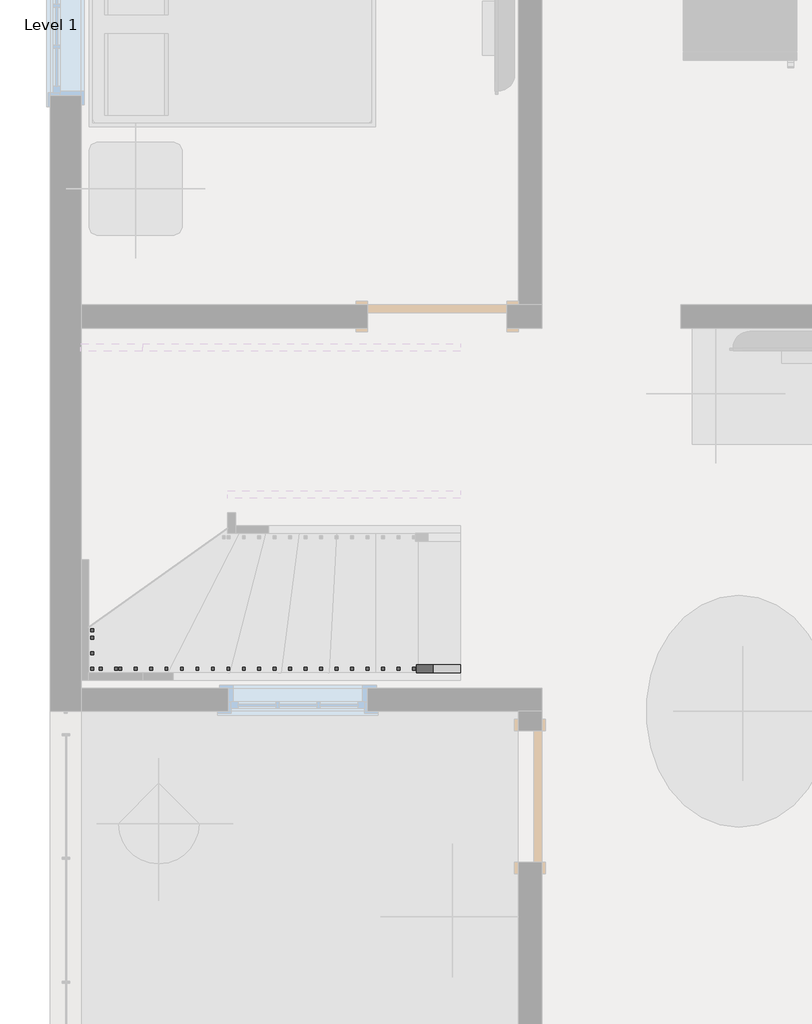
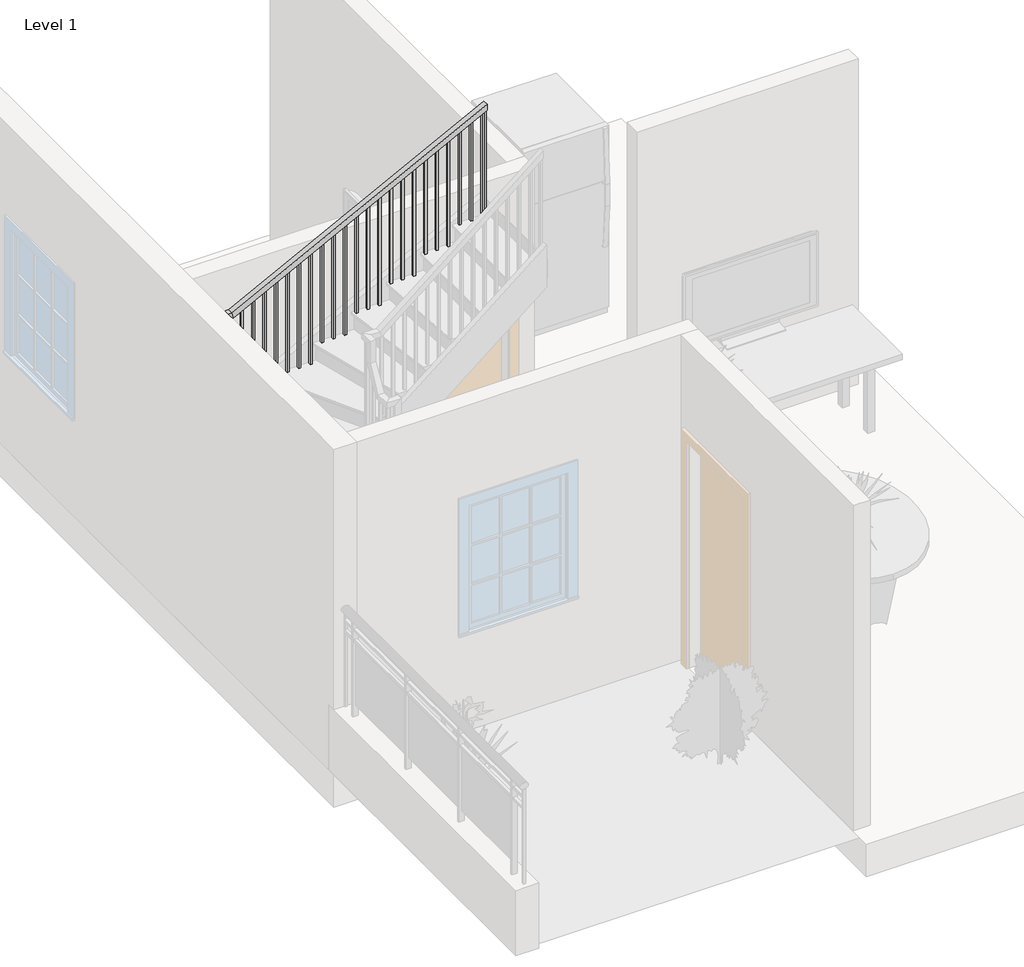
# One storey, part 2 of 3: 1 railing.
"""IFC4 building model written with IfcOpenShell, lengths in millimetres."""

from ifc_helpers import new_model, si_unit, frame, origin, place, context, project, spatial, polyline, outline, extrude, faceted_brep, element, save

model = new_model("IFC4")

# Units and contexts
model_context = context("Model", 3, world=origin())
ifc_project = project(units=[si_unit("LENGTHUNIT", "METRE", prefix="MILLI")], contexts=[model_context])

# Site, building, storey
site = spatial("IfcSite", under=ifc_project)
building = spatial("IfcBuilding", under=site)
storey = spatial("IfcBuildingStorey", under=building, Name="Level 1", Elevation=0.0)

# Railing
placement = place(None, origin())
element("IfcRailing", 1, ObjectType="Handrail - Rectangular", at=placement, inside=storey, context=model_context, shape_type="SolidModel", body=[
    faceted_brep([(-14092.4170266, 6866.6465295, 1109.0771751), (-14092.4170266, 6866.6465295, 1051.9280057), (-14092.4170266, 6917.4465295, 1051.9280057), (-14092.4170266, 6917.4465295, 1109.0771751), (-16352.3988831, 6866.6465295, 2273.7644996), (-16364.7189344, 6866.6465295, 2222.9644996), (-16364.7189344, 6917.4465295, 2222.9644996), (-16352.3988831, 6917.4465295, 2273.7644996), (-16534.5487184, 6866.6465295, 2273.7644996), (-16534.5487184, 6866.6465295, 2222.9644996), (-16483.7487184, 6917.4465295, 2222.9644996), (-16483.7487184, 6917.4465295, 2273.7644996), (-16534.5487184, 7143.8004821, 2273.7644996), (-16534.5487184, 7151.7510582, 2222.9644996), (-16483.7487184, 7151.7510582, 2222.9644996), (-16483.7487184, 7143.8004821, 2273.7644996), (-16534.5487184, 8697.6925768, 2772.3688337), (-16534.5487184, 8705.643153, 2721.5688337), (-16483.7487184, 8705.643153, 2721.5688337), (-16483.7487184, 8697.6925768, 2772.3688337), (-16534.5487184, 8974.8465295, 2772.3688337), (-16534.5487184, 8974.8465295, 2721.5688337), (-16483.7487184, 8924.0465295, 2721.5688337), (-16483.7487184, 8924.0465295, 2772.3688337), (-16352.3988831, 8974.8465295, 2772.3688337), (-16340.0788318, 8974.8465295, 2721.5688337), (-16340.0788318, 8924.0465295, 2721.5688337), (-16352.3988831, 8924.0465295, 2772.3688337), (-14092.4170266, 8974.8465295, 3937.0561582), (-14092.4170266, 8924.0465295, 3937.0561582), (-14092.4170266, 8924.0465295, 3879.9069889), (-14092.4170266, 8974.8465295, 3879.9069889)], [[[0, 1, 2, 3]], [[1, 0, 4, 5]], [[2, 1, 5, 6]], [[3, 2, 6, 7]], [[0, 3, 7, 4]], [[5, 4, 8, 9]], [[6, 5, 9, 10]], [[7, 6, 10, 11]], [[4, 7, 11, 8]], [[9, 8, 12, 13]], [[10, 9, 13, 14]], [[11, 10, 14, 15]], [[8, 11, 15, 12]], [[13, 12, 16, 17]], [[14, 13, 17, 18]], [[15, 14, 18, 19]], [[12, 15, 19, 16]], [[17, 16, 20, 21]], [[18, 17, 21, 22]], [[19, 18, 22, 23]], [[16, 19, 23, 20]], [[21, 20, 24, 25]], [[22, 21, 25, 26]], [[23, 22, 26, 27]], [[20, 23, 27, 24]], [[28, 29, 30, 31]], [[25, 24, 28, 31]], [[26, 25, 31, 30]], [[27, 26, 30, 29]], [[24, 27, 29, 28]]]),
    extrude(outline(polyline([(3862.2268642, -14126.7238831), (2878.6666667, -14126.7238831), (2878.6666667, -14107.6738831), (3872.0443296, -14107.6738831), (3862.2268642, -14126.7238831)])), frame((0.0, 8939.9215295, 0.0), z_axis=(0.0, 1.0, 0.0), x_axis=(0.0, 0.0, 1.0)), (0.0, 0.0, 1.0), 19.05),
    extrude(outline(polyline([(3809.8670491, -14228.3238831), (2878.6666667, -14228.3238831), (2878.6666667, -14209.2738831), (3819.6845145, -14209.2738831), (3809.8670491, -14228.3238831)])), frame((0.0, 8939.9215295, 0.0), z_axis=(0.0, 1.0, 0.0), x_axis=(0.0, 0.0, 1.0)), (0.0, 0.0, 1.0), 19.05),
    extrude(outline(polyline([(3757.507234, -14329.9238831), (2878.6666667, -14329.9238831), (2878.6666667, -14310.8738831), (3767.3246993, -14310.8738831), (3757.507234, -14329.9238831)])), frame((0.0, 8939.9215295, 0.0), z_axis=(0.0, 1.0, 0.0), x_axis=(0.0, 0.0, 1.0)), (0.0, 0.0, 1.0), 19.05),
    extrude(outline(polyline([(3705.1474189, -14431.5238831), (2709.3333333, -14431.5238831), (2709.3333333, -14412.4738831), (3714.9648842, -14412.4738831), (3705.1474189, -14431.5238831)])), frame((0.0, 8939.9215295, 0.0), z_axis=(0.0, 1.0, 0.0), x_axis=(0.0, 0.0, 1.0)), (0.0, 0.0, 1.0), 19.05),
    extrude(outline(polyline([(3652.7876038, -14533.1238831), (2709.3333333, -14533.1238831), (2709.3333333, -14514.0738831), (3662.6050691, -14514.0738831), (3652.7876038, -14533.1238831)])), frame((0.0, 8939.9215295, 0.0), z_axis=(0.0, 1.0, 0.0), x_axis=(0.0, 0.0, 1.0)), (0.0, 0.0, 1.0), 19.05),
    extrude(outline(polyline([(3600.4277887, -14634.7238831), (2709.3333333, -14634.7238831), (2709.3333333, -14615.6738831), (3610.245254, -14615.6738831), (3600.4277887, -14634.7238831)])), frame((0.0, 8939.9215295, 0.0), z_axis=(0.0, 1.0, 0.0), x_axis=(0.0, 0.0, 1.0)), (0.0, 0.0, 1.0), 19.05),
    extrude(outline(polyline([(3548.0679735, -14736.3238831), (2540.0, -14736.3238831), (2540.0, -14717.2738831), (3557.8854389, -14717.2738831), (3548.0679735, -14736.3238831)])), frame((0.0, 8939.9215295, 0.0), z_axis=(0.0, 1.0, 0.0), x_axis=(0.0, 0.0, 1.0)), (0.0, 0.0, 1.0), 19.05),
    extrude(outline(polyline([(3495.7081584, -14837.9238831), (2540.0, -14837.9238831), (2540.0, -14818.8738831), (3505.5256238, -14818.8738831), (3495.7081584, -14837.9238831)])), frame((0.0, 8939.9215295, 0.0), z_axis=(0.0, 1.0, 0.0), x_axis=(0.0, 0.0, 1.0)), (0.0, 0.0, 1.0), 19.05),
    extrude(outline(polyline([(3443.3483433, -14939.5238831), (2540.0, -14939.5238831), (2540.0, -14920.4738831), (3453.1658086, -14920.4738831), (3443.3483433, -14939.5238831)])), frame((0.0, 8939.9215295, 0.0), z_axis=(0.0, 1.0, 0.0), x_axis=(0.0, 0.0, 1.0)), (0.0, 0.0, 1.0), 19.05),
    extrude(outline(polyline([(3390.9885282, -15041.1238831), (2370.6666667, -15041.1238831), (2370.6666667, -15022.0738831), (3400.8059935, -15022.0738831), (3390.9885282, -15041.1238831)])), frame((0.0, 8939.9215295, 0.0), z_axis=(0.0, 1.0, 0.0), x_axis=(0.0, 0.0, 1.0)), (0.0, 0.0, 1.0), 19.05),
    extrude(outline(polyline([(3338.6287131, -15142.7238831), (2370.6666667, -15142.7238831), (2370.6666667, -15123.6738831), (3348.4461784, -15123.6738831), (3338.6287131, -15142.7238831)])), frame((0.0, 8939.9215295, 0.0), z_axis=(0.0, 1.0, 0.0), x_axis=(0.0, 0.0, 1.0)), (0.0, 0.0, 1.0), 19.05),
    extrude(outline(polyline([(3286.268898, -15244.3238831), (2370.6666667, -15244.3238831), (2370.6666667, -15225.2738831), (3296.0863633, -15225.2738831), (3286.268898, -15244.3238831)])), frame((0.0, 8939.9215295, 0.0), z_axis=(0.0, 1.0, 0.0), x_axis=(0.0, 0.0, 1.0)), (0.0, 0.0, 1.0), 19.05),
    extrude(outline(polyline([(3233.9090828, -15345.9238831), (2201.3333333, -15345.9238831), (2201.3333333, -15326.8738831), (3243.7265482, -15326.8738831), (3233.9090828, -15345.9238831)])), frame((0.0, 8939.9215295, 0.0), z_axis=(0.0, 1.0, 0.0), x_axis=(0.0, 0.0, 1.0)), (0.0, 0.0, 1.0), 19.05),
    extrude(outline(polyline([(3181.5492677, -15447.5238831), (2201.3333333, -15447.5238831), (2201.3333333, -15428.4738831), (3191.3667331, -15428.4738831), (3181.5492677, -15447.5238831)])), frame((0.0, 8939.9215295, 0.0), z_axis=(0.0, 1.0, 0.0), x_axis=(0.0, 0.0, 1.0)), (0.0, 0.0, 1.0), 19.05),
    extrude(outline(polyline([(3129.1894526, -15549.1238831), (2201.3333333, -15549.1238831), (2201.3333333, -15530.0738831), (3139.0069179, -15530.0738831), (3129.1894526, -15549.1238831)])), frame((0.0, 8939.9215295, 0.0), z_axis=(0.0, 1.0, 0.0), x_axis=(0.0, 0.0, 1.0)), (0.0, 0.0, 1.0), 19.05),
    extrude(outline(polyline([(3076.8296375, -15650.7238831), (2032.0, -15650.7238831), (2032.0, -15631.6738831), (3086.6471028, -15631.6738831), (3076.8296375, -15650.7238831)])), frame((0.0, 8939.9215295, 0.0), z_axis=(0.0, 1.0, 0.0), x_axis=(0.0, 0.0, 1.0)), (0.0, 0.0, 1.0), 19.05),
    extrude(outline(polyline([(3024.4698224, -15752.3238831), (2032.0, -15752.3238831), (2032.0, -15733.2738831), (3034.2872877, -15733.2738831), (3024.4698224, -15752.3238831)])), frame((0.0, 8939.9215295, 0.0), z_axis=(0.0, 1.0, 0.0), x_axis=(0.0, 0.0, 1.0)), (0.0, 0.0, 1.0), 19.05),
    extrude(outline(polyline([(2972.1100073, -15853.9238831), (2032.0, -15853.9238831), (2032.0, -15834.8738831), (2981.9274726, -15834.8738831), (2972.1100073, -15853.9238831)])), frame((0.0, 8939.9215295, 0.0), z_axis=(0.0, 1.0, 0.0), x_axis=(0.0, 0.0, 1.0)), (0.0, 0.0, 1.0), 19.05),
    extrude(outline(polyline([(2919.7501921, -15955.5238831), (2032.0, -15955.5238831), (2032.0, -15936.4738831), (2929.5676575, -15936.4738831), (2919.7501921, -15955.5238831)])), frame((0.0, 8939.9215295, 0.0), z_axis=(0.0, 1.0, 0.0), x_axis=(0.0, 0.0, 1.0)), (0.0, 0.0, 1.0), 19.05),
    extrude(outline(polyline([(2867.390377, -16057.1238831), (1862.6666667, -16057.1238831), (1862.6666667, -16038.0738831), (2877.2078424, -16038.0738831), (2867.390377, -16057.1238831)])), frame((0.0, 8939.9215295, 0.0), z_axis=(0.0, 1.0, 0.0), x_axis=(0.0, 0.0, 1.0)), (0.0, 0.0, 1.0), 19.05),
    extrude(outline(polyline([(2815.0305619, -16158.7238831), (1862.6666667, -16158.7238831), (1862.6666667, -16139.6738831), (2824.8480272, -16139.6738831), (2815.0305619, -16158.7238831)])), frame((0.0, 8939.9215295, 0.0), z_axis=(0.0, 1.0, 0.0), x_axis=(0.0, 0.0, 1.0)), (0.0, 0.0, 1.0), 19.05),
    extrude(outline(polyline([(2762.6707468, -16260.3238831), (1862.6666667, -16260.3238831), (1862.6666667, -16241.2738831), (2772.4882121, -16241.2738831), (2762.6707468, -16260.3238831)])), frame((0.0, 8939.9215295, 0.0), z_axis=(0.0, 1.0, 0.0), x_axis=(0.0, 0.0, 1.0)), (0.0, 0.0, 1.0), 19.05),
    extrude(outline(polyline([(-16417.0737184, 8958.9715295), (-16398.0237184, 8958.9715295), (-16398.0237184, 8939.9215295), (-16417.0737184, 8939.9215295), (-16417.0737184, 8958.9715295)])), frame((0.0, 0.0, 1862.6666667), z_axis=(0.0, 0.0, 1.0), x_axis=(1.0, 0.0, 0.0)), (0.0, 0.0, 1.0), 858.902167),
    extrude(outline(polyline([(-16518.6737184, 8891.3675768), (-16518.6737184, 8910.4175768), (-16499.6237184, 8910.4175768), (-16499.6237184, 8891.3675768), (-16518.6737184, 8891.3675768)])), frame((0.0, 0.0, 1862.6666667), z_axis=(0.0, 0.0, 1.0), x_axis=(1.0, 0.0, 0.0)), (0.0, 0.0, 1.0), 858.902167),
    extrude(outline(polyline([(-16518.6737184, 8789.7675768), (-16518.6737184, 8808.8175768), (-16499.6237184, 8808.8175768), (-16499.6237184, 8789.7675768), (-16518.6737184, 8789.7675768)])), frame((0.0, 0.0, 1862.6666667), z_axis=(0.0, 0.0, 1.0), x_axis=(1.0, 0.0, 0.0)), (0.0, 0.0, 1.0), 858.902167),
    extrude(outline(polyline([(8677.3254821, 2712.4824155), (8677.3254821, 1693.3333333), (8658.2754821, 1693.3333333), (8658.2754821, 2706.3697564), (8677.3254821, 2712.4824155)])), frame((-16518.6737184, 0.0, 0.0), z_axis=(1.0, 0.0, 0.0), x_axis=(0.0, 1.0, 0.0)), (0.0, 0.0, 1.0), 19.05),
    extrude(outline(polyline([(8575.7254821, 2679.8815673), (8575.7254821, 1693.3333333), (8556.6754821, 1693.3333333), (8556.6754821, 2673.7689082), (8575.7254821, 2679.8815673)])), frame((-16518.6737184, 0.0, 0.0), z_axis=(1.0, 0.0, 0.0), x_axis=(0.0, 1.0, 0.0)), (0.0, 0.0, 1.0), 19.05),
    extrude(outline(polyline([(8474.1254821, 2647.280719), (8474.1254821, 1693.3333333), (8455.0754821, 1693.3333333), (8455.0754821, 2641.16806), (8474.1254821, 2647.280719)])), frame((-16518.6737184, 0.0, 0.0), z_axis=(1.0, 0.0, 0.0), x_axis=(0.0, 1.0, 0.0)), (0.0, 0.0, 1.0), 19.05),
    extrude(outline(polyline([(8372.5254821, 2614.6798708), (8372.5254821, 1693.3333333), (8353.4754821, 1693.3333333), (8353.4754821, 2608.5672118), (8372.5254821, 2614.6798708)])), frame((-16518.6737184, 0.0, 0.0), z_axis=(1.0, 0.0, 0.0), x_axis=(0.0, 1.0, 0.0)), (0.0, 0.0, 1.0), 19.05),
    extrude(outline(polyline([(8270.9254821, 2582.0790226), (8270.9254821, 1693.3333333), (8251.8754821, 1693.3333333), (8251.8754821, 2575.9663635), (8270.9254821, 2582.0790226)])), frame((-16518.6737184, 0.0, 0.0), z_axis=(1.0, 0.0, 0.0), x_axis=(0.0, 1.0, 0.0)), (0.0, 0.0, 1.0), 19.05),
    extrude(outline(polyline([(8169.3254821, 2549.4781744), (8169.3254821, 1693.3333333), (8150.2754821, 1693.3333333), (8150.2754821, 2543.3655153), (8169.3254821, 2549.4781744)])), frame((-16518.6737184, 0.0, 0.0), z_axis=(1.0, 0.0, 0.0), x_axis=(0.0, 1.0, 0.0)), (0.0, 0.0, 1.0), 19.05),
    extrude(outline(polyline([(8067.7254821, 2516.8773261), (8067.7254821, 1524.0), (8048.6754821, 1524.0), (8048.6754821, 2510.7646671), (8067.7254821, 2516.8773261)])), frame((-16518.6737184, 0.0, 0.0), z_axis=(1.0, 0.0, 0.0), x_axis=(0.0, 1.0, 0.0)), (0.0, 0.0, 1.0), 19.05),
    extrude(outline(polyline([(7966.1254821, 2484.2764779), (7966.1254821, 1524.0), (7947.0754821, 1524.0), (7947.0754821, 2478.1638189), (7966.1254821, 2484.2764779)])), frame((-16518.6737184, 0.0, 0.0), z_axis=(1.0, 0.0, 0.0), x_axis=(0.0, 1.0, 0.0)), (0.0, 0.0, 1.0), 19.05),
    extrude(outline(polyline([(7864.5254821, 2451.6756297), (7864.5254821, 1524.0), (7845.4754821, 1524.0), (7845.4754821, 2445.5629706), (7864.5254821, 2451.6756297)])), frame((-16518.6737184, 0.0, 0.0), z_axis=(1.0, 0.0, 0.0), x_axis=(0.0, 1.0, 0.0)), (0.0, 0.0, 1.0), 19.05),
    extrude(outline(polyline([(7762.9254821, 2419.0747814), (7762.9254821, 1524.0), (7743.8754821, 1524.0), (7743.8754821, 2412.9621224), (7762.9254821, 2419.0747814)])), frame((-16518.6737184, 0.0, 0.0), z_axis=(1.0, 0.0, 0.0), x_axis=(0.0, 1.0, 0.0)), (0.0, 0.0, 1.0), 19.05),
    extrude(outline(polyline([(7661.3254821, 2386.4739332), (7661.3254821, 1354.6666667), (7642.2754821, 1354.6666667), (7642.2754821, 2380.3612742), (7661.3254821, 2386.4739332)])), frame((-16518.6737184, 0.0, 0.0), z_axis=(1.0, 0.0, 0.0), x_axis=(0.0, 1.0, 0.0)), (0.0, 0.0, 1.0), 19.05),
    extrude(outline(polyline([(7559.7254821, 2353.873085), (7559.7254821, 1354.6666667), (7540.6754821, 1354.6666667), (7540.6754821, 2347.7604259), (7559.7254821, 2353.873085)])), frame((-16518.6737184, 0.0, 0.0), z_axis=(1.0, 0.0, 0.0), x_axis=(0.0, 1.0, 0.0)), (0.0, 0.0, 1.0), 19.05),
    extrude(outline(polyline([(7458.1254821, 2321.2722368), (7458.1254821, 1354.6666667), (7439.0754821, 1354.6666667), (7439.0754821, 2315.1595777), (7458.1254821, 2321.2722368)])), frame((-16518.6737184, 0.0, 0.0), z_axis=(1.0, 0.0, 0.0), x_axis=(0.0, 1.0, 0.0)), (0.0, 0.0, 1.0), 19.05),
    extrude(outline(polyline([(7356.5254821, 2288.6713885), (7356.5254821, 1354.6666667), (7337.4754821, 1354.6666667), (7337.4754821, 2282.5587295), (7356.5254821, 2288.6713885)])), frame((-16518.6737184, 0.0, 0.0), z_axis=(1.0, 0.0, 0.0), x_axis=(0.0, 1.0, 0.0)), (0.0, 0.0, 1.0), 19.05),
    extrude(outline(polyline([(7254.9254821, 2256.0705403), (7254.9254821, 1354.6666667), (7235.8754821, 1354.6666667), (7235.8754821, 2249.9578813), (7254.9254821, 2256.0705403)])), frame((-16518.6737184, 0.0, 0.0), z_axis=(1.0, 0.0, 0.0), x_axis=(0.0, 1.0, 0.0)), (0.0, 0.0, 1.0), 19.05),
    extrude(outline(polyline([(-16518.6737184, 7085.7215295), (-16518.6737184, 7104.7715295), (-16499.6237184, 7104.7715295), (-16499.6237184, 7085.7215295), (-16518.6737184, 7085.7215295)])), frame((0.0, 0.0, 1185.3333333), z_axis=(0.0, 0.0, 1.0), x_axis=(1.0, 0.0, 0.0)), (0.0, 0.0, 1.0), 1037.6311663),
    extrude(outline(polyline([(-16518.6737184, 6984.1215295), (-16518.6737184, 7003.1715295), (-16499.6237184, 7003.1715295), (-16499.6237184, 6984.1215295), (-16518.6737184, 6984.1215295)])), frame((0.0, 0.0, 1185.3333333), z_axis=(0.0, 0.0, 1.0), x_axis=(1.0, 0.0, 0.0)), (0.0, 0.0, 1.0), 1037.6311663),
    extrude(outline(polyline([(-16444.4738831, 6882.5215295), (-16463.5238831, 6882.5215295), (-16463.5238831, 6901.5715295), (-16444.4738831, 6901.5715295), (-16444.4738831, 6882.5215295)])), frame((0.0, 0.0, 1185.3333333), z_axis=(0.0, 0.0, 1.0), x_axis=(1.0, 0.0, 0.0)), (0.0, 0.0, 1.0), 1037.6311663),
    extrude(outline(polyline([(2208.752671, -16337.1420266), (1185.3333333, -16337.1420266), (1185.3333333, -16318.0920266), (2198.9352056, -16318.0920266), (2208.752671, -16337.1420266)])), frame((0.0, 6882.5215295, 0.0), z_axis=(0.0, 1.0, 0.0), x_axis=(0.0, 0.0, 1.0)), (0.0, 0.0, 1.0), 19.05),
    extrude(outline(polyline([(2156.3928558, -16235.5420266), (1185.3333333, -16235.5420266), (1185.3333333, -16216.4920266), (2146.5753905, -16216.4920266), (2156.3928558, -16235.5420266)])), frame((0.0, 6882.5215295, 0.0), z_axis=(0.0, 1.0, 0.0), x_axis=(0.0, 0.0, 1.0)), (0.0, 0.0, 1.0), 19.05),
    extrude(outline(polyline([(2104.0330407, -16133.9420266), (1185.3333333, -16133.9420266), (1185.3333333, -16114.8920266), (2094.2155754, -16114.8920266), (2104.0330407, -16133.9420266)])), frame((0.0, 6882.5215295, 0.0), z_axis=(0.0, 1.0, 0.0), x_axis=(0.0, 0.0, 1.0)), (0.0, 0.0, 1.0), 19.05),
    extrude(outline(polyline([(2051.6732256, -16032.3420266), (1185.3333333, -16032.3420266), (1185.3333333, -16013.2920266), (2041.8557603, -16013.2920266), (2051.6732256, -16032.3420266)])), frame((0.0, 6882.5215295, 0.0), z_axis=(0.0, 1.0, 0.0), x_axis=(0.0, 0.0, 1.0)), (0.0, 0.0, 1.0), 19.05),
    extrude(outline(polyline([(1999.3134105, -15930.7420266), (1016.0, -15930.7420266), (1016.0, -15911.6920266), (1989.4959452, -15911.6920266), (1999.3134105, -15930.7420266)])), frame((0.0, 6882.5215295, 0.0), z_axis=(0.0, 1.0, 0.0), x_axis=(0.0, 0.0, 1.0)), (0.0, 0.0, 1.0), 19.05),
    extrude(outline(polyline([(1946.9535954, -15829.1420266), (1016.0, -15829.1420266), (1016.0, -15810.0920266), (1937.13613, -15810.0920266), (1946.9535954, -15829.1420266)])), frame((0.0, 6882.5215295, 0.0), z_axis=(0.0, 1.0, 0.0), x_axis=(0.0, 0.0, 1.0)), (0.0, 0.0, 1.0), 19.05),
    extrude(outline(polyline([(1894.5937803, -15727.5420266), (1016.0, -15727.5420266), (1016.0, -15708.4920266), (1884.7763149, -15708.4920266), (1894.5937803, -15727.5420266)])), frame((0.0, 6882.5215295, 0.0), z_axis=(0.0, 1.0, 0.0), x_axis=(0.0, 0.0, 1.0)), (0.0, 0.0, 1.0), 19.05),
    extrude(outline(polyline([(1842.2339651, -15625.9420266), (1016.0, -15625.9420266), (1016.0, -15606.8920266), (1832.4164998, -15606.8920266), (1842.2339651, -15625.9420266)])), frame((0.0, 6882.5215295, 0.0), z_axis=(0.0, 1.0, 0.0), x_axis=(0.0, 0.0, 1.0)), (0.0, 0.0, 1.0), 19.05),
    extrude(outline(polyline([(1789.87415, -15524.3420266), (846.6666667, -15524.3420266), (846.6666667, -15505.2920266), (1780.0566847, -15505.2920266), (1789.87415, -15524.3420266)])), frame((0.0, 6882.5215295, 0.0), z_axis=(0.0, 1.0, 0.0), x_axis=(0.0, 0.0, 1.0)), (0.0, 0.0, 1.0), 19.05),
    extrude(outline(polyline([(1737.5143349, -15422.7420266), (846.6666667, -15422.7420266), (846.6666667, -15403.6920266), (1727.6968696, -15403.6920266), (1737.5143349, -15422.7420266)])), frame((0.0, 6882.5215295, 0.0), z_axis=(0.0, 1.0, 0.0), x_axis=(0.0, 0.0, 1.0)), (0.0, 0.0, 1.0), 19.05),
    extrude(outline(polyline([(1685.1545198, -15321.1420266), (846.6666667, -15321.1420266), (846.6666667, -15302.0920266), (1675.3370545, -15302.0920266), (1685.1545198, -15321.1420266)])), frame((0.0, 6882.5215295, 0.0), z_axis=(0.0, 1.0, 0.0), x_axis=(0.0, 0.0, 1.0)), (0.0, 0.0, 1.0), 19.05),
    extrude(outline(polyline([(1632.7947047, -15219.5420266), (677.3333333, -15219.5420266), (677.3333333, -15200.4920266), (1622.9772393, -15200.4920266), (1632.7947047, -15219.5420266)])), frame((0.0, 6882.5215295, 0.0), z_axis=(0.0, 1.0, 0.0), x_axis=(0.0, 0.0, 1.0)), (0.0, 0.0, 1.0), 19.05),
    extrude(outline(polyline([(1580.4348896, -15117.9420266), (677.3333333, -15117.9420266), (677.3333333, -15098.8920266), (1570.6174242, -15098.8920266), (1580.4348896, -15117.9420266)])), frame((0.0, 6882.5215295, 0.0), z_axis=(0.0, 1.0, 0.0), x_axis=(0.0, 0.0, 1.0)), (0.0, 0.0, 1.0), 19.05),
    extrude(outline(polyline([(1528.0750744, -15016.3420266), (677.3333333, -15016.3420266), (677.3333333, -14997.2920266), (1518.2576091, -14997.2920266), (1528.0750744, -15016.3420266)])), frame((0.0, 6882.5215295, 0.0), z_axis=(0.0, 1.0, 0.0), x_axis=(0.0, 0.0, 1.0)), (0.0, 0.0, 1.0), 19.05),
    extrude(outline(polyline([(1475.7152593, -14914.7420266), (508.0, -14914.7420266), (508.0, -14895.6920266), (1465.897794, -14895.6920266), (1475.7152593, -14914.7420266)])), frame((0.0, 6882.5215295, 0.0), z_axis=(0.0, 1.0, 0.0), x_axis=(0.0, 0.0, 1.0)), (0.0, 0.0, 1.0), 19.05),
    extrude(outline(polyline([(1423.3554442, -14813.1420266), (508.0, -14813.1420266), (508.0, -14794.0920266), (1413.5379789, -14794.0920266), (1423.3554442, -14813.1420266)])), frame((0.0, 6882.5215295, 0.0), z_axis=(0.0, 1.0, 0.0), x_axis=(0.0, 0.0, 1.0)), (0.0, 0.0, 1.0), 19.05),
    extrude(outline(polyline([(1370.9956291, -14711.5420266), (508.0, -14711.5420266), (508.0, -14692.4920266), (1361.1781638, -14692.4920266), (1370.9956291, -14711.5420266)])), frame((0.0, 6882.5215295, 0.0), z_axis=(0.0, 1.0, 0.0), x_axis=(0.0, 0.0, 1.0)), (0.0, 0.0, 1.0), 19.05),
    extrude(outline(polyline([(1318.635814, -14609.9420266), (338.6666667, -14609.9420266), (338.6666667, -14590.8920266), (1308.8183486, -14590.8920266), (1318.635814, -14609.9420266)])), frame((0.0, 6882.5215295, 0.0), z_axis=(0.0, 1.0, 0.0), x_axis=(0.0, 0.0, 1.0)), (0.0, 0.0, 1.0), 19.05),
    extrude(outline(polyline([(1266.2759989, -14508.3420266), (338.6666667, -14508.3420266), (338.6666667, -14489.2920266), (1256.4585335, -14489.2920266), (1266.2759989, -14508.3420266)])), frame((0.0, 6882.5215295, 0.0), z_axis=(0.0, 1.0, 0.0), x_axis=(0.0, 0.0, 1.0)), (0.0, 0.0, 1.0), 19.05),
    extrude(outline(polyline([(1213.9161837, -14406.7420266), (338.6666667, -14406.7420266), (338.6666667, -14387.6920266), (1204.0987184, -14387.6920266), (1213.9161837, -14406.7420266)])), frame((0.0, 6882.5215295, 0.0), z_axis=(0.0, 1.0, 0.0), x_axis=(0.0, 0.0, 1.0)), (0.0, 0.0, 1.0), 19.05),
    extrude(outline(polyline([(1161.5563686, -14305.1420266), (169.3333333, -14305.1420266), (169.3333333, -14286.0920266), (1151.7389033, -14286.0920266), (1161.5563686, -14305.1420266)])), frame((0.0, 6882.5215295, 0.0), z_axis=(0.0, 1.0, 0.0), x_axis=(0.0, 0.0, 1.0)), (0.0, 0.0, 1.0), 19.05),
    extrude(outline(polyline([(1109.1965535, -14203.5420266), (169.3333333, -14203.5420266), (169.3333333, -14184.4920266), (1099.3790882, -14184.4920266), (1109.1965535, -14203.5420266)])), frame((0.0, 6882.5215295, 0.0), z_axis=(0.0, 1.0, 0.0), x_axis=(0.0, 0.0, 1.0)), (0.0, 0.0, 1.0), 19.05),
    extrude(outline(polyline([(-16361.9238831, 8958.9715295), (-16342.8738831, 8958.9715295), (-16342.8738831, 8939.9215295), (-16361.9238831, 8939.9215295), (-16361.9238831, 8958.9715295)])), frame((0.0, 0.0, 1862.6666667), z_axis=(0.0, 0.0, 1.0), x_axis=(1.0, 0.0, 0.0)), (0.0, 0.0, 1.0), 858.902167),
    extrude(outline(polyline([(-16518.6737184, 8939.9215295), (-16518.6737184, 8958.9715295), (-16499.6237184, 8958.9715295), (-16499.6237184, 8939.9215295), (-16518.6737184, 8939.9215295)])), frame((0.0, 0.0, 1862.6666667), z_axis=(0.0, 0.0, 1.0), x_axis=(1.0, 0.0, 0.0)), (0.0, 0.0, 1.0), 858.902167),
    extrude(outline(polyline([(8707.2175768, 2722.0740262), (8707.2175768, 1862.6666667), (8688.1675768, 1862.6666667), (8688.1675768, 2715.9613671), (8707.2175768, 2722.0740262)])), frame((-16518.6737184, 0.0, 0.0), z_axis=(1.0, 0.0, 0.0), x_axis=(0.0, 1.0, 0.0)), (0.0, 0.0, 1.0), 19.05),
    extrude(outline(polyline([(-16518.6737184, 7134.2754821), (-16518.6737184, 7153.3254821), (-16499.6237184, 7153.3254821), (-16499.6237184, 7134.2754821), (-16518.6737184, 7134.2754821)])), frame((0.0, 0.0, 1185.3333333), z_axis=(0.0, 0.0, 1.0), x_axis=(1.0, 0.0, 0.0)), (0.0, 0.0, 1.0), 1037.6311663),
    extrude(outline(polyline([(-16499.6237184, 6882.5215295), (-16518.6737184, 6882.5215295), (-16518.6737184, 6901.5715295), (-16499.6237184, 6901.5715295), (-16499.6237184, 6882.5215295)])), frame((0.0, 0.0, 1185.3333333), z_axis=(0.0, 0.0, 1.0), x_axis=(1.0, 0.0, 0.0)), (0.0, 0.0, 1.0), 1037.6311663),
    extrude(outline(polyline([(2221.5240629, -16361.9238831), (1185.3333333, -16361.9238831), (1185.3333333, -16342.8738831), (2211.7065976, -16342.8738831), (2221.5240629, -16361.9238831)])), frame((0.0, 6882.5215295, 0.0), z_axis=(0.0, 1.0, 0.0), x_axis=(0.0, 0.0, 1.0)), (0.0, 0.0, 1.0), 19.05),
    extrude(outline(polyline([(3870.0895235, -14111.4670266), (2878.6666667, -14111.4670266), (2878.6666667, -14092.4170266), (3879.9069889, -14092.4170266), (3870.0895235, -14111.4670266)])), frame((0.0, 8939.9215295, 0.0), z_axis=(0.0, 1.0, 0.0), x_axis=(0.0, 0.0, 1.0)), (0.0, 0.0, 1.0), 19.05),
    extrude(outline(polyline([(1061.7454711, -14111.4670266), (169.3333333, -14111.4670266), (169.3333333, -14092.4170266), (1051.9280057, -14092.4170266), (1061.7454711, -14111.4670266)])), frame((0.0, 6882.5215295, 0.0), z_axis=(0.0, 1.0, 0.0), x_axis=(0.0, 0.0, 1.0)), (0.0, 0.0, 1.0), 19.05),
])

save(model, "model.ifc")

# Revit data of these elements
# Type "Handrail - Rectangular"
#   Assembly Code = "C2010400"
#   built-in parameter 1008612 = 0.0416667 (stored number, unit not read)
#   built-in parameter 1008611 = 0.0416667 (stored number, unit not read)
#   built-in parameter 1008609 = 0.333333 (stored number, unit not read)
#   built-in parameter 1008604 = 0.166667 (stored number, unit not read)
#   built-in parameter 1008603 = 0.166667 (stored number, unit not read)
#   Railing Height = 3' - 0"
#   built-in parameter 1008630 = 2
#   built-in parameter 1008610 = 2
#   built-in parameter 1008618 = Baluster - Square : 3/4"
# Element 1 (IfcRailing, "Handrail - Rectangular")
#   Phase Created = New Construction
